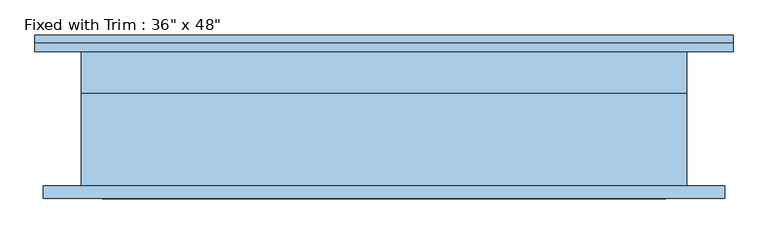
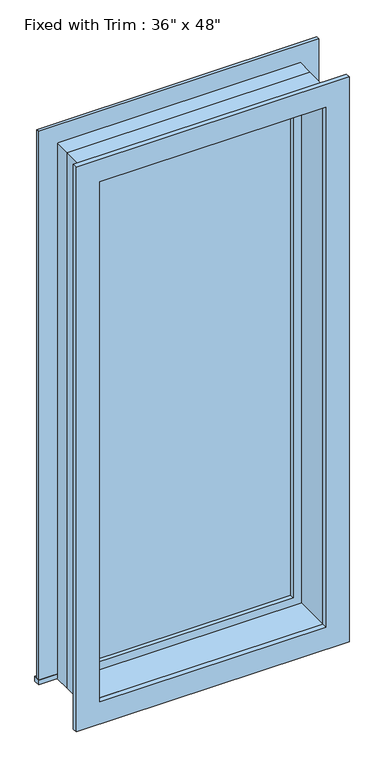
"""IFC4 building model written with IfcOpenShell, lengths in millimetres: window geometry."""

from ifc_helpers import new_model, si_unit, frame, origin, place, context, project, spatial, polyline, outline, extrude, source, transform, mapped, element, save


def window_4ca78fb8(model_context):
    return source(origin(), model_context, "Body", "SweptSolid", [
        extrude(outline(polyline([(-565.15, 127.0), (488.95, 127.0), (488.95, 101.6), (-565.15, 101.6), (-565.15, 127.0)])), frame((0.0, 0.0, 914.4), z_axis=(0.0, 0.0, 1.0), x_axis=(1.0, 0.0, 0.0)), (0.0, 0.0, 1.0), 19.05),
        extrude(outline(polyline([(3028.95, -476.25), (3028.95, 400.05), (933.45, 400.05), (933.45, 488.95), (3117.85, 488.95), (3117.85, -565.15), (933.45, -565.15), (933.45, -476.25), (3028.95, -476.25)])), frame((0.0, 101.6, 0.0), z_axis=(0.0, 1.0, 0.0), x_axis=(0.0, 0.0, 1.0)), (0.0, 0.0, 1.0), 12.7),
        extrude(outline(polyline([(3105.15, 476.25), (3105.15, -552.45), (857.25, -552.45), (857.25, 476.25), (3105.15, 476.25)]), holes=[polyline([(3016.25, 387.35), (946.15, 387.35), (946.15, -463.55), (3016.25, -463.55), (3016.25, 387.35)])]), frame((0.0, -120.65, 0.0), z_axis=(0.0, 1.0, 0.0), x_axis=(0.0, 0.0, 1.0)), (0.0, 0.0, 1.0), 19.05),
        extrude(outline(polyline([(355.6, 53.975), (-431.8, 53.975), (-431.8, 66.675), (355.6, 66.675), (355.6, 53.975)])), frame((0.0, 0.0, 977.9), z_axis=(0.0, 0.0, 1.0), x_axis=(1.0, 0.0, 0.0)), (0.0, 0.0, 1.0), 2006.6),
        extrude(outline(polyline([(3028.95, -476.25), (933.45, -476.25), (933.45, 400.05), (3028.95, 400.05), (3028.95, -476.25)]), holes=[polyline([(2984.5, -431.8), (2984.5, 355.6), (977.9, 355.6), (977.9, -431.8), (2984.5, -431.8)])]), frame((0.0, 38.1, 0.0), z_axis=(0.0, 1.0, 0.0), x_axis=(0.0, 0.0, 1.0)), (0.0, 0.0, 1.0), 44.45),
        extrude(outline(polyline([(3048.0, -495.3), (914.4, -495.3), (914.4, 419.1), (3048.0, 419.1), (3048.0, -495.3)]), holes=[polyline([(3016.25, -463.55), (3016.25, 387.35), (946.15, 387.35), (946.15, -463.55), (3016.25, -463.55)])]), frame((0.0, -101.6, 0.0), z_axis=(0.0, 1.0, 0.0), x_axis=(0.0, 0.0, 1.0)), (0.0, 0.0, 1.0), 139.7),
        extrude(outline(polyline([(3048.0, 419.1), (3048.0, -495.3), (914.4, -495.3), (914.4, 419.1), (3048.0, 419.1)]), holes=[polyline([(3028.95, 400.05), (933.45, 400.05), (933.45, -476.25), (3028.95, -476.25), (3028.95, 400.05)])]), frame((0.0, 38.1, 0.0), z_axis=(0.0, 1.0, 0.0), x_axis=(0.0, 0.0, 1.0)), (0.0, 0.0, 1.0), 63.5),
    ])


if __name__ == "__main__":
    model = new_model("IFC4")
    model_context = context("Model", 3, world=origin())
    ifc_project = project(units=[si_unit("LENGTHUNIT", "METRE", prefix="MILLI")], contexts=[model_context])
    site = spatial("IfcSite", under=ifc_project)
    building = spatial("IfcBuilding", under=site)
    placement = place(None, origin())
    window_shape = window_4ca78fb8(model_context)
    element("IfcWindow", 1, ObjectType="Fixed with Trim : 36\" x 48\"", at=placement, inside=building, context=model_context, shape_type="MappedRepresentation", body=[
        mapped(window_shape, transform((0.0, 0.0, 0.0), x_axis=(1.0, 0.0, 0.0), y_axis=(0.0, 1.0, 0.0), z_axis=(0.0, 0.0, 1.0))),
    ])
    save(model, "model.ifc")

# Revit data of these elements
# Type "Fixed with Trim : 36\" x 48\""
#   Type Mark = "10"
#   Construction Type Id = "GSP4R"
#   Assembly Code = "B2020100"
#   Analytic Construction = "1/8 in Pilkington single glazing"
#   Visual Light Transmittance = 0.9
#   Solar Heat Gain Coefficient = 0.78
#   Heat Transfer Coefficient (U) = 0.6496 BTU/(h·ft²·°F)
#   Height = 7' - 0"
#   Default Sill Height = 3' - 0"
#   Trim Projection - Ext. = 0' - 0 1/2"
#   Trim Projection - Int. = 0' - 0 3/4"
#   Trim Width - Exterior = 0' - 3 1/2"
#   Trim Width - Interior = 0' - 3 1/2"
#   Width = 3' - 0"
#   Window Inset = 0' - 0 3/4"
#   Define Thermal Properties by = 1
#   Glass Pane Material = Glass
#   Sash Material = Sash
#   Trim Exterior Material = Trim
#   Trim Interior Material = Trim
#   Wall Closure = (empty or 0)
# Element 1 (IfcWindow, "Fixed with Trim : 36\" x 48\"")
#   Materials on its faces: "Sash", "Trim", "Glass"
# Materials
#   "Glass": class "Glass", colour RGB 0 128 192, transparency 0.75, Description = "Soda Lime Glass", Cost = 0
#   "Sash": class "Wood", colour RGB 224 178 126, transparency 0
#   "Trim": class "Wood", colour RGB 224 178 126, transparency 0
